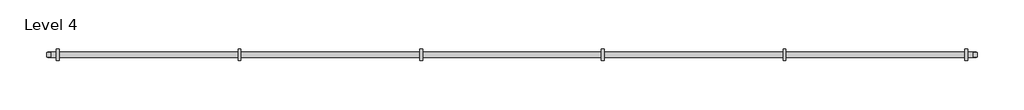
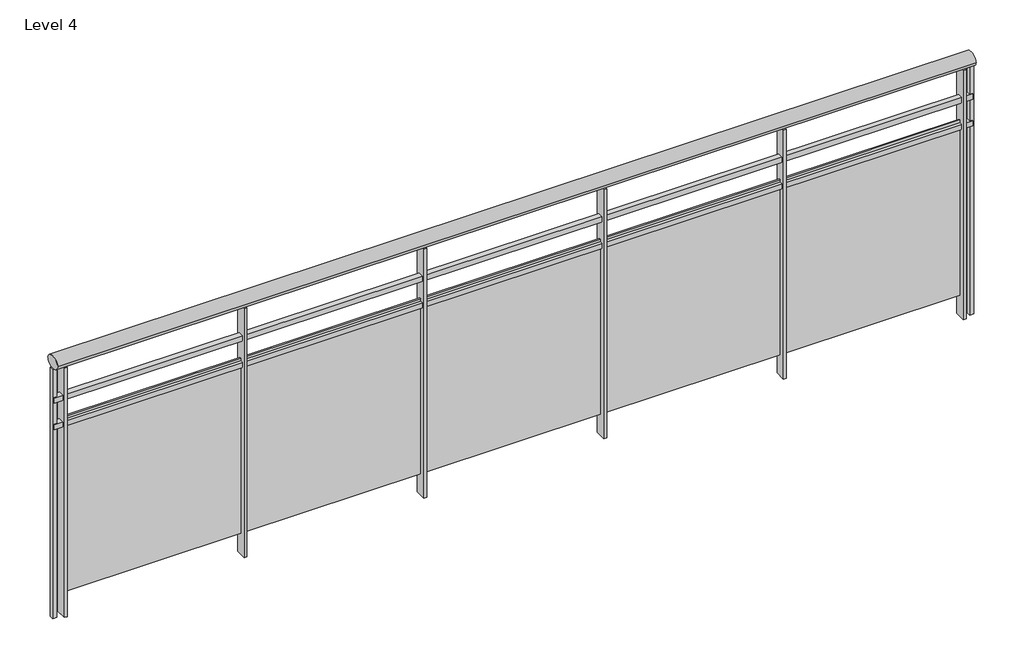
# One storey: 1 railing.
"""IFC4 building model written with IfcOpenShell, lengths in millimetres."""

from ifc_helpers import new_model, si_unit, point, frame, origin, place, context, project, spatial, polyline, ellipse_curve, trimmed, outline, extrude, element, save
from ifc_brep_helpers import plane_surface, extruded_surface, advanced_brep

model = new_model("IFC4")

# Units and contexts
model_context = context("Model", 3, world=origin())
ifc_project = project(units=[si_unit("LENGTHUNIT", "METRE", prefix="MILLI")], contexts=[model_context])

# Site, building, storey
site = spatial("IfcSite", under=ifc_project)
building = spatial("IfcBuilding", under=site)
storey = spatial("IfcBuildingStorey", under=building, Name="Level 4", Elevation=9601.2)

# Railing
placement = place(None, origin())
element("IfcRailing", 1, ObjectType="Glass Panel - Bottom Fill", at=placement, inside=storey, context=model_context, shape_type="SolidModel", body=[
    advanced_brep(
    [(-5729.1673724, -5829.5544725, 10820.4), (-5729.1673724, -5905.7544725, 10820.4), (-1576.8982041, -5829.5544725, 10820.4), (-1576.8982041, -5905.7544725, 10820.4)],
    [
        (0, 1, ellipse_curve(frame((-5729.1673724, -5867.6544725, 10820.4), z_axis=(-1.0, 0.0, 0.0), x_axis=(0.0, -1.0, 0.0)), 38.1, 28.575)),
        (1, 0, ellipse_curve(frame((-5729.1673724, -5867.6544725, 10820.4), z_axis=(-1.0, 0.0, 0.0), x_axis=(0.0, -1.0, 0.0)), 38.1, 28.575)),
        (2, 3, ellipse_curve(frame((-1576.8982041, -5867.6544725, 10820.4), z_axis=(1.0, 0.0, 0.0), x_axis=(0.0, -1.0, 0.0)), 38.1, 28.575)),
        (3, 2, ellipse_curve(frame((-1576.8982041, -5867.6544725, 10820.4), z_axis=(1.0, 0.0, 0.0), x_axis=(0.0, -1.0, 0.0)), 38.1, 28.575)),
        (0, 2),
        (3, 1),
    ],
    [
        plane_surface(frame((-5729.1673724, -5867.6544725, 10820.4), z_axis=(-1.0, 0.0, 0.0), x_axis=(0.0, 1.0, 0.0))),
        plane_surface(frame((-1576.8982041, -5867.6544725, 10820.4), z_axis=(1.0, 0.0, 0.0), x_axis=(0.0, 1.0, 0.0))),
        extruded_surface(trimmed(ellipse_curve(frame((-1576.8982041, -5867.6544725, 10820.4), z_axis=(-1.0, 0.0, 0.0), x_axis=(0.0, -1.0, 0.0)), 38.1, 28.575), [point((-1576.8982041, -5829.5544725, 10820.4))], [point((-1576.8982041, -5905.7544725, 10820.4))], True, "CARTESIAN"), (-4152.2691683, 0.0, 0.0), 4152.2691683),
        extruded_surface(trimmed(ellipse_curve(frame((-1576.8982041, -5867.6544725, 10820.4), z_axis=(-1.0, 0.0, 0.0), x_axis=(0.0, -1.0, 0.0)), 38.1, 28.575), [point((-1576.8982041, -5905.7544725, 10820.4))], [point((-1576.8982041, -5829.5544725, 10820.4))], True, "CARTESIAN"), (-4152.2691683, 0.0, 0.0), 4152.2691683),
    ],
    [
        (0, [[1, 2]]),
        (1, [[3, 4]]),
        (2, [[-1, 5, -4, 6]]),
        (3, [[-2, -6, -3, -5]]),
    ],
),
    extrude(outline(polyline([(-5729.1673724, -5880.3544725), (-5729.1673724, -5854.9544725), (-1576.8982041, -5854.9544725), (-1576.8982041, -5880.3544725), (-5729.1673724, -5880.3544725)])), frame((0.0, 0.0, 10629.9), z_axis=(0.0, 0.0, 1.0), x_axis=(1.0, 0.0, 0.0)), (0.0, 0.0, 1.0), 25.4),
    extrude(outline(polyline([(-5729.1673724, -5880.3544725), (-5729.1673724, -5854.9544725), (-1576.8982041, -5854.9544725), (-1576.8982041, -5880.3544725), (-5729.1673724, -5880.3544725)])), frame((0.0, 0.0, 10502.9), z_axis=(0.0, 0.0, 1.0), x_axis=(1.0, 0.0, 0.0)), (0.0, 0.0, 1.0), 25.4),
    extrude(outline(polyline([(-1627.3827882, -5893.0544725), (-1627.3827882, -5842.2544725), (-1614.6827882, -5842.2544725), (-1614.6827882, -5893.0544725), (-1627.3827882, -5893.0544725)])), frame((0.0, 0.0, 9601.2), z_axis=(0.0, 0.0, 1.0), x_axis=(1.0, 0.0, 0.0)), (0.0, 0.0, 1.0), 1190.625),
    extrude(outline(polyline([(-2433.8327882, -5861.1193155), (-1621.0327882, -5861.1193155), (-1621.0327882, -5867.4693155), (-2433.8327882, -5867.4693155), (-2433.8327882, -5861.1193155)])), frame((0.0, 0.0, 9702.8), z_axis=(0.0, 0.0, 1.0), x_axis=(1.0, 0.0, 0.0)), (0.0, 0.0, 1.0), 838.2),
    extrude(outline(polyline([(-2440.1827882, -5893.0544725), (-2440.1827882, -5842.2544725), (-2427.4827882, -5842.2544725), (-2427.4827882, -5893.0544725), (-2440.1827882, -5893.0544725)])), frame((0.0, 0.0, 9601.2), z_axis=(0.0, 0.0, 1.0), x_axis=(1.0, 0.0, 0.0)), (0.0, 0.0, 1.0), 1190.625),
    extrude(outline(polyline([(-3246.6327882, -5861.1193155), (-2433.8327882, -5861.1193155), (-2433.8327882, -5867.4693155), (-3246.6327882, -5867.4693155), (-3246.6327882, -5861.1193155)])), frame((0.0, 0.0, 9702.8), z_axis=(0.0, 0.0, 1.0), x_axis=(1.0, 0.0, 0.0)), (0.0, 0.0, 1.0), 838.2),
    extrude(outline(polyline([(-3252.9827882, -5893.0544725), (-3252.9827882, -5842.2544725), (-3240.2827882, -5842.2544725), (-3240.2827882, -5893.0544725), (-3252.9827882, -5893.0544725)])), frame((0.0, 0.0, 9601.2), z_axis=(0.0, 0.0, 1.0), x_axis=(1.0, 0.0, 0.0)), (0.0, 0.0, 1.0), 1190.625),
    extrude(outline(polyline([(-4059.4327882, -5861.1193155), (-3246.6327882, -5861.1193155), (-3246.6327882, -5867.4693155), (-4059.4327882, -5867.4693155), (-4059.4327882, -5861.1193155)])), frame((0.0, 0.0, 9702.8), z_axis=(0.0, 0.0, 1.0), x_axis=(1.0, 0.0, 0.0)), (0.0, 0.0, 1.0), 838.2),
    extrude(outline(polyline([(-4065.7827882, -5893.0544725), (-4065.7827882, -5842.2544725), (-4053.0827882, -5842.2544725), (-4053.0827882, -5893.0544725), (-4065.7827882, -5893.0544725)])), frame((0.0, 0.0, 9601.2), z_axis=(0.0, 0.0, 1.0), x_axis=(1.0, 0.0, 0.0)), (0.0, 0.0, 1.0), 1190.625),
    extrude(outline(polyline([(-4872.2327882, -5861.1193155), (-4059.4327882, -5861.1193155), (-4059.4327882, -5867.4693155), (-4872.2327882, -5867.4693155), (-4872.2327882, -5861.1193155)])), frame((0.0, 0.0, 9702.8), z_axis=(0.0, 0.0, 1.0), x_axis=(1.0, 0.0, 0.0)), (0.0, 0.0, 1.0), 838.2),
    extrude(outline(polyline([(-4878.5827882, -5893.0544725), (-4878.5827882, -5842.2544725), (-4865.8827882, -5842.2544725), (-4865.8827882, -5893.0544725), (-4878.5827882, -5893.0544725)])), frame((0.0, 0.0, 9601.2), z_axis=(0.0, 0.0, 1.0), x_axis=(1.0, 0.0, 0.0)), (0.0, 0.0, 1.0), 1190.625),
    extrude(outline(polyline([(-5685.0327882, -5861.1193155), (-4872.2327882, -5861.1193155), (-4872.2327882, -5867.4693155), (-5685.0327882, -5867.4693155), (-5685.0327882, -5861.1193155)])), frame((0.0, 0.0, 9702.8), z_axis=(0.0, 0.0, 1.0), x_axis=(1.0, 0.0, 0.0)), (0.0, 0.0, 1.0), 838.2),
    extrude(outline(polyline([(-5691.3827882, -5893.0544725), (-5691.3827882, -5842.2544725), (-5678.6827882, -5842.2544725), (-5678.6827882, -5893.0544725), (-5691.3827882, -5893.0544725)])), frame((0.0, 0.0, 9601.2), z_axis=(0.0, 0.0, 1.0), x_axis=(1.0, 0.0, 0.0)), (0.0, 0.0, 1.0), 1190.625),
    extrude(outline(polyline([(-1589.5982041, -5877.1794725), (-1589.5982041, -5858.1294725), (-1570.5482041, -5858.1294725), (-1570.5482041, -5877.1794725), (-1589.5982041, -5877.1794725)])), frame((0.0, 0.0, 9601.2), z_axis=(0.0, 0.0, 1.0), x_axis=(1.0, 0.0, 0.0)), (0.0, 0.0, 1.0), 1190.625),
    extrude(outline(polyline([(-5735.5173724, -5877.1794725), (-5735.5173724, -5858.1294725), (-5716.4673724, -5858.1294725), (-5716.4673724, -5877.1794725), (-5735.5173724, -5877.1794725)])), frame((0.0, 0.0, 9601.2), z_axis=(0.0, 0.0, 1.0), x_axis=(1.0, 0.0, 0.0)), (0.0, 0.0, 1.0), 1190.625),
])

save(model, "model.ifc")

# Revit data of these elements
# Type "Glass Panel - Bottom Fill"
#   Assembly Code = "C2010400"
#   built-in parameter 1008612 = 0.0416667 (stored number, unit not read)
#   built-in parameter 1008611 = 0.0416667 (stored number, unit not read)
#   built-in parameter 1008609 = 0.333333 (stored number, unit not read)
#   built-in parameter 1008604 = 0.166667 (stored number, unit not read)
#   built-in parameter 1008603 = 0.166667 (stored number, unit not read)
#   Railing Height = 4' - 0"
#   built-in parameter 1008630 = 2
#   built-in parameter 1008610 = 2
#   built-in parameter 1008618 = Baluster - Square : 3/4"
# Element 1 (IfcRailing, "Glass Panel - Bottom Fill")
#   Phase Created = New Construction
#   Materials on its faces: "Glass"
# Materials
#   "Glass": class "Glass", colour RGB 0 128 192, transparency 0.75, Description = "Soda Lime Glass", Cost = 0
